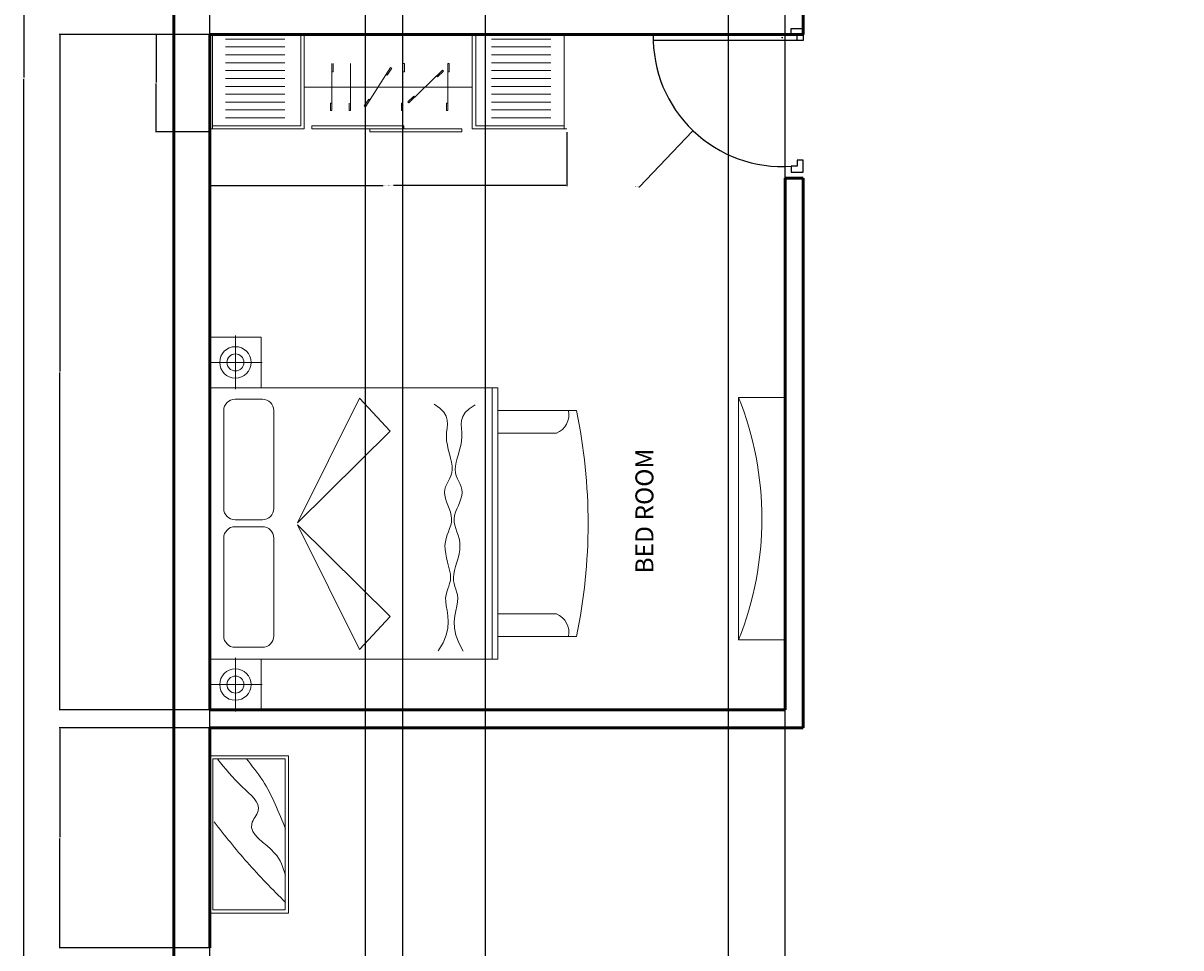
# Model space of a CAD drawing. Units: inches. Extents: x 1865 to 2541, y 1997 to 2759.
# Tile 2 of 11: x 1866 to 2155, y 2174 to 2405. Entities that reach past the tile are written whole.
import ezdxf

# ---------------------------------------------------------------- set-up
doc = ezdxf.new("R2010")
doc.units = ezdxf.units.IN
for name, color, linetype, lineweight in [('A-ANNO-DIMS', 2, 'Continuous', 18), ('A-AREA-IDEN', 4, 'Continuous', 18), ('A-FURN', 8, 'Continuous', 13), ('A-WALL', 7, 'Continuous', 50), ('BED', 42, 'Continuous', 13), ('CUPBOARD', 61, 'Continuous', 18), ('DOOR', 1, 'Continuous', 25), ('TV', 3, 'Continuous', 18)]:
    doc.layers.add(name, color=color, linetype=linetype, lineweight=lineweight)
doc.styles.get("Standard").update_dxf_attribs({"font": 'arial.ttf'})
doc.dimstyles.get("Standard").update_dxf_attribs({"dimtxt": 0.18, "dimasz": 0.18, "dimexe": 0.18, "dimexo": 0.0625, "dimgap": 0.09, "dimtad": 0, "dimtih": 1, "dimtoh": 1, "dimdec": 4, "dimzin": 0, "dimdsep": 46, "dimtxsty": 'Standard', "dimcen": 0.09, "dimadec": 0, "dimazin": 0, "dimtfac": 1, "dimtdec": 4, "dimtofl": 0, "dimtmove": 0, "dimatfit": 3, "dimfxl": 1, "dimtolj": 1, "dimtzin": 0, "dimarcsym": 0})

# ---------------------------------------------------------------- blocks, each defined once
blk = doc.blocks.new('A$C4F543DC7')
for p, q in [((0.013, 3.35, -0.169), (3.313, 3.35, -0.169)), ((0.463, 3.35, -0.169), (0.013, 3.35, -0.169)), ((0.013, 2.896, -0.169), (0.013, 3.35, -0.169)), ((0.013, 3.35, -0.169), (0.013, 2.896, -0.169)), ((0.238, 3.123, -0.439), (0.238, 3.361, -0.439)), ((0.463, 3.35, -0.169), (0.463, 0.8, -0.169)), ((2.863, 3.35, -0.169), (0.463, 3.35, -0.169)), ((0.463, 2.896, -0.169), (0.463, 3.35, -0.169)), ((2.863, 0.8, -0.169), (2.863, 3.35, -0.169)), ((2.863, 3.35, -0.169), (3.313, 3.35, -0.169)), ((2.863, 2.896, -0.169), (2.863, 3.35, -0.169)), ((3.089, 3.123, -0.439), (3.089, 3.361, -0.439)), ((3.313, 3.35, -0.169), (3.313, 2.896, -0.169)), ((3.313, 3.35, -0.169), (3.313, 2.896, -0.169)), ((1.535, 3.226, -0.169), (0.668, 3.226, -0.169)), ((2.664, 3.226, -0.169), (1.797, 3.226, -0.169)), ((0.238, 3.123, -0.439), (0, 3.123, -0.439)), ((0.238, 3.123, -0.439), (0.476, 3.123, -0.439)), ((0.238, 3.123, -0.439), (0.238, 2.885, -0.439)), ((0.568, 3.126, -0.169), (0.568, 2.884, -0.169)), ((1.635, 2.884, -0.169), (1.635, 3.126, -0.169)), ((1.697, 3.126, -0.169), (1.697, 2.884, -0.169)), ((2.764, 2.884, -0.169), (2.764, 3.126, -0.169)), ((3.089, 3.123, -0.439), (2.851, 3.123, -0.439)), ((3.089, 3.123, -0.439), (3.089, 2.885, -0.439)), ((3.089, 3.123, -0.439), (3.327, 3.123, -0.439)), ((0.463, 2.896, -0.169), (0.013, 2.896, -0.169)), ((0.013, 2.896, -0.169), (0.463, 2.896, -0.169)), ((0.463, 0.8, -0.169), (0.463, 2.896, -0.169)), ((2.863, 2.896, -0.169), (2.863, 0.8, -0.169)), ((3.313, 2.896, -0.169), (2.863, 2.896, -0.169)), ((3.313, 2.896, -0.169), (2.863, 2.896, -0.169)), ((0.668, 2.784, -0.169), (1.535, 2.784, -0.169)), ((1.797, 2.784, -0.169), (2.664, 2.784, -0.169)), ((1.653, 2.573, -0.169), (0.55, 2.025, -0.169)), ((0.841, 1.752, -0.169), (1.653, 2.573, -0.169)), ((2.481, 1.752, -0.169), (1.669, 2.573, -0.169)), ((1.669, 2.573, -0.169), (2.772, 2.025, -0.169)), ((0.55, 2.025, -0.169), (0.841, 1.752, -0.169)), ((2.772, 2.025, -0.169), (2.481, 1.752, -0.169)), ((2.683, 1.312, -0.169), (2.718, 1.364, -0.169)), ((0.537, 1.327, -0.169), (0.609, 1.284, -0.169)), ((0.609, 1.284, -0.169), (0.676, 1.257, -0.169)), ((0.676, 1.257, -0.169), (0.737, 1.243, -0.169)), ((0.737, 1.243, -0.169), (0.794, 1.239, -0.169)), ((0.794, 1.239, -0.169), (0.846, 1.242, -0.169)), ((0.846, 1.242, -0.169), (0.893, 1.249, -0.169)), ((0.893, 1.249, -0.169), (0.935, 1.256, -0.169)), ((0.935, 1.256, -0.169), (0.972, 1.261, -0.169)), ((0.972, 1.261, -0.169), (1.004, 1.262, -0.169)), ((1.004, 1.262, -0.169), (1.033, 1.258, -0.169)), ((1.033, 1.258, -0.169), (1.06, 1.251, -0.169)), ((1.06, 1.251, -0.169), (1.084, 1.242, -0.169)), ((1.084, 1.242, -0.169), (1.108, 1.234, -0.169)), ((1.108, 1.234, -0.169), (1.132, 1.226, -0.169)), ((1.25, 1.226, -0.169), (1.285, 1.235, -0.169)), ((1.285, 1.235, -0.169), (1.322, 1.244, -0.169)), ((1.322, 1.244, -0.169), (1.359, 1.253, -0.169)), ((1.359, 1.253, -0.169), (1.396, 1.261, -0.169)), ((1.396, 1.261, -0.169), (1.433, 1.266, -0.169)), ((1.433, 1.266, -0.169), (1.468, 1.268, -0.169)), ((1.468, 1.268, -0.169), (1.501, 1.264, -0.169)), ((1.501, 1.264, -0.169), (1.532, 1.257, -0.169)), ((1.532, 1.257, -0.169), (1.562, 1.247, -0.169)), ((1.562, 1.247, -0.169), (1.591, 1.237, -0.169)), ((1.591, 1.237, -0.169), (1.62, 1.226, -0.169)), ((1.765, 1.22, -0.169), (1.795, 1.23, -0.169)), ((1.795, 1.23, -0.169), (1.826, 1.242, -0.169)), ((1.826, 1.242, -0.169), (1.856, 1.253, -0.169)), ((1.856, 1.253, -0.169), (1.885, 1.263, -0.169)), ((1.885, 1.263, -0.169), (1.913, 1.27, -0.169)), ((1.913, 1.27, -0.169), (1.94, 1.272, -0.169)), ((1.94, 1.272, -0.169), (1.965, 1.269, -0.169)), ((1.965, 1.269, -0.169), (1.989, 1.262, -0.169)), ((1.989, 1.262, -0.169), (2.012, 1.251, -0.169)), ((2.012, 1.251, -0.169), (2.036, 1.239, -0.169)), ((2.036, 1.239, -0.169), (2.06, 1.227, -0.169)), ((2.279, 1.228, -0.169), (2.317, 1.238, -0.169)), ((2.317, 1.238, -0.169), (2.356, 1.246, -0.169)), ((2.356, 1.246, -0.169), (2.394, 1.253, -0.169)), ((2.394, 1.253, -0.169), (2.433, 1.255, -0.169)), ((2.433, 1.255, -0.169), (2.47, 1.253, -0.169)), ((2.47, 1.253, -0.169), (2.506, 1.249, -0.169)), ((2.506, 1.249, -0.169), (2.542, 1.246, -0.169)), ((2.542, 1.246, -0.169), (2.578, 1.248, -0.169)), ((2.578, 1.248, -0.169), (2.613, 1.257, -0.169)), ((2.613, 1.257, -0.169), (2.648, 1.277, -0.169)), ((2.648, 1.277, -0.169), (2.683, 1.312, -0.169)), ((0.533, 1.105, -0.169), (0.607, 1.146, -0.169)), ((0.607, 1.146, -0.169), (0.674, 1.171, -0.169)), ((0.674, 1.171, -0.169), (0.736, 1.183, -0.169)), ((0.736, 1.183, -0.169), (0.793, 1.185, -0.169)), ((0.793, 1.185, -0.169), (0.845, 1.18, -0.169)), ((0.845, 1.18, -0.169), (0.891, 1.172, -0.169)), ((0.891, 1.172, -0.169), (0.933, 1.163, -0.169)), ((0.933, 1.163, -0.169), (0.97, 1.156, -0.169)), ((0.97, 1.156, -0.169), (1.003, 1.155, -0.169)), ((1.003, 1.155, -0.169), (1.032, 1.158, -0.169)), ((1.032, 1.158, -0.169), (1.058, 1.164, -0.169)), ((1.058, 1.164, -0.169), (1.083, 1.172, -0.169)), ((1.083, 1.172, -0.169), (1.107, 1.18, -0.169)), ((1.107, 1.18, -0.169), (1.132, 1.187, -0.169)), ((1.132, 1.226, -0.169), (1.158, 1.22, -0.169)), ((1.132, 1.187, -0.169), (1.157, 1.192, -0.169)), ((1.157, 1.192, -0.169), (1.185, 1.193, -0.169)), ((1.158, 1.22, -0.169), (1.185, 1.218, -0.169)), ((1.185, 1.218, -0.169), (1.216, 1.22, -0.169)), ((1.185, 1.193, -0.169), (1.216, 1.19, -0.169)), ((1.216, 1.22, -0.169), (1.25, 1.226, -0.169)), ((1.216, 1.19, -0.169), (1.249, 1.183, -0.169)), ((1.249, 1.183, -0.169), (1.284, 1.173, -0.169)), ((1.284, 1.173, -0.169), (1.321, 1.163, -0.169)), ((1.321, 1.163, -0.169), (1.358, 1.152, -0.169)), ((1.358, 1.152, -0.169), (1.394, 1.143, -0.169)), ((1.394, 1.143, -0.169), (1.431, 1.137, -0.169)), ((1.431, 1.137, -0.169), (1.466, 1.135, -0.169)), ((1.466, 1.135, -0.169), (1.499, 1.137, -0.169)), ((1.499, 1.137, -0.169), (1.531, 1.143, -0.169)), ((1.531, 1.143, -0.169), (1.561, 1.152, -0.169)), ((1.561, 1.152, -0.169), (1.59, 1.162, -0.169)), ((1.59, 1.162, -0.169), (1.619, 1.172, -0.169)), ((1.619, 1.172, -0.169), (1.648, 1.18, -0.169)), ((1.62, 1.226, -0.169), (1.648, 1.217, -0.169)), ((1.648, 1.217, -0.169), (1.676, 1.211, -0.169)), ((1.648, 1.18, -0.169), (1.676, 1.185, -0.169)), ((1.676, 1.211, -0.169), (1.705, 1.209, -0.169)), ((1.676, 1.185, -0.169), (1.705, 1.186, -0.169)), ((1.705, 1.209, -0.169), (1.735, 1.212, -0.169)), ((1.705, 1.186, -0.169), (1.734, 1.182, -0.169)), ((1.734, 1.182, -0.169), (1.764, 1.173, -0.169)), ((1.735, 1.212, -0.169), (1.765, 1.22, -0.169)), ((1.764, 1.173, -0.169), (1.794, 1.162, -0.169)), ((1.794, 1.162, -0.169), (1.824, 1.149, -0.169)), ((1.824, 1.149, -0.169), (1.854, 1.137, -0.169)), ((1.854, 1.137, -0.169), (1.883, 1.126, -0.169)), ((1.987, 1.124, -0.169), (2.011, 1.134, -0.169)), ((2.011, 1.134, -0.169), (2.034, 1.145, -0.169)), ((2.034, 1.145, -0.169), (2.059, 1.157, -0.169)), ((2.059, 1.157, -0.169), (2.084, 1.167, -0.169)), ((2.06, 1.227, -0.169), (2.085, 1.216, -0.169)), ((2.084, 1.167, -0.169), (2.111, 1.174, -0.169)), ((2.085, 1.216, -0.169), (2.112, 1.208, -0.169)), ((2.111, 1.174, -0.169), (2.14, 1.177, -0.169)), ((2.112, 1.208, -0.169), (2.141, 1.204, -0.169)), ((2.14, 1.177, -0.169), (2.172, 1.175, -0.169)), ((2.141, 1.204, -0.169), (2.172, 1.205, -0.169)), ((2.172, 1.205, -0.169), (2.206, 1.21, -0.169)), ((2.172, 1.175, -0.169), (2.206, 1.169, -0.169)), ((2.206, 1.21, -0.169), (2.242, 1.218, -0.169)), ((2.206, 1.169, -0.169), (2.241, 1.16, -0.169)), ((2.241, 1.16, -0.169), (2.278, 1.149, -0.169)), ((2.242, 1.218, -0.169), (2.279, 1.228, -0.169)), ((2.278, 1.149, -0.169), (2.316, 1.138, -0.169)), ((2.316, 1.138, -0.169), (2.354, 1.128, -0.169)), ((2.354, 1.128, -0.169), (2.392, 1.121, -0.169)), ((1.883, 1.126, -0.169), (1.911, 1.119, -0.169)), ((1.911, 1.119, -0.169), (1.937, 1.115, -0.169)), ((1.937, 1.115, -0.169), (1.963, 1.118, -0.169)), ((1.963, 1.118, -0.169), (1.987, 1.124, -0.169)), ((2.392, 1.121, -0.169), (2.43, 1.117, -0.169)), ((2.43, 1.117, -0.169), (2.468, 1.118, -0.169)), ((2.468, 1.118, -0.169), (2.504, 1.121, -0.169)), ((2.504, 1.121, -0.169), (2.54, 1.123, -0.169)), ((2.54, 1.123, -0.169), (2.576, 1.12, -0.169)), ((2.576, 1.12, -0.169), (2.611, 1.109, -0.169)), ((2.611, 1.109, -0.169), (2.645, 1.088, -0.169)), ((2.645, 1.088, -0.169), (2.679, 1.052, -0.169)), ((2.679, 1.052, -0.169), (2.712, 0.999, -0.169)), ((0.463, 0.85, -0.169), (2.863, 0.85, -0.169)), ((0.463, 0.8, -0.169), (2.863, 0.8, -0.169)), ((0.663, 0.8, -0.169), (0.463, 0.8, -0.169)), ((0.663, 0.8, -0.169), (2.663, 0.8, -0.169)), ((0.663, 0.104, -0.169), (0.663, 0.8, -0.169)), ((0.663, 0.104, -0.169), (0.663, 0.8, -0.169)), ((0.863, 0.281, -0.169), (0.863, 0.8, -0.169)), ((2.463, 0.8, -0.169), (2.463, 0.281, -0.169)), ((2.863, 0.8, -0.169), (2.663, 0.8, -0.169)), ((2.663, 0.8, -0.169), (2.663, 0.104, -0.169)), ((2.663, 0.8, -0.169), (2.663, 0.104, -0.169))]:
    blk.add_line(p, q)
for centre, radius in [((0.238, 3.123, -0.439), 0.139), ((0.238, 3.123, -0.439), 0.075), ((3.089, 3.123, -0.439), 0.139), ((3.089, 3.123, -0.439), 0.075)]:
    blk.add_circle(centre, radius)
for centre, radius, start, end in [((0.668, 3.126, -0.169), 0.1, 90, 180), ((1.535, 3.126, -0.169), 0.1, 0, 90), ((1.797, 3.126, -0.169), 0.1, 90, 180), ((2.664, 3.126, -0.169), 0.1, 0, 90), ((0.668, 2.884, -0.169), 0.1, 180, 270), ((1.535, 2.884, -0.169), 0.1, 270, 0), ((1.797, 2.884, -0.169), 0.1, 180, 270), ((2.664, 2.884, -0.169), 0.1, 270, 0), ((0.699, 0.347, -0.169), 0.177, 258.2616, 338.032), ((2.627, 0.347, -0.169), 0.177, 201.968, 281.7384), ((1.663, 4.86, -0.169), 4.86, 258.1252, 281.8748), ((1.663, 4.86, -0.169), 4.86, 258.1252, 281.8748)]:
    blk.add_arc(centre, radius, start, end)
blk = doc.blocks.new('A$C34930FF8')
at = {"ltscale": 0.05}
for p, q in [((0, 2252.4), (0, 16.8)), ((600, 2252.4), (0, 2252.4)), ((185.4, 1513), (185.4, 1521.5)), ((227.1, 1479.2), (233.2, 1485.2)), ((237.7, 1513), (237.7, 1521.5)), ((436.7, 1513), (436.7, 1504.4)), ((482.5, 1513), (482.5, 1504.4)), ((263.6, 1441.7), (269.7, 1447.7)), ((398.2, 1303.6), (392.1, 1297.6)), ((434.8, 1266.1), (428.7, 1260.1)), ((185.4, 1229.1), (185.4, 1237.7)), ((237.7, 1229.1), (237.7, 1237.7)), ((436.7, 1228.2), (436.7, 1219.7)), ((482.5, 1228.2), (482.5, 1219.7)), ((209.5, 1150.1), (214.1, 1157.3)), ((253.5, 1121.8), (258.1, 1129)), ((415.3, 1017.6), (410.6, 1010.5)), ((459.3, 989.3), (454.7, 982.1)), ((482.5, 894.9), (482.5, 886.3)), ((237.7, 775.3), (237.7, 783.9)), ((436.7, 775.3), (436.7, 766.8)), ((482.5, 775.3), (482.5, 766.8)), ((600, 16.8), (0, 16.8))]:
    blk.add_line(p, q, dxfattribs=at)
for p, q in [((580, 1690.9), (580, 2252.4)), ((600, 1669.3), (600, 2269.3)), ((30, 1790.9), (30, 2169.3)), ((80, 1790.9), (80, 2169.3)), ((130, 1790.9), (130, 2169.3)), ((180, 1790.9), (180, 2169.3)), ((230, 1790.9), (230, 2169.3)), ((280, 1790.9), (280, 2169.3)), ((330, 1790.9), (330, 2169.3)), ((380, 1790.9), (380, 2169.3)), ((430, 1790.9), (430, 2169.3)), ((480, 1790.9), (480, 2169.3)), ((530, 1790.9), (530, 2169.3)), ((580, 1690.9), (0, 1690.9)), ((600, 1669.3), (0, 1669.3)), ((335.4, 1666.1), (335.4, 603.1)), ((600, 1603.3), (620, 1603.3)), ((600, 1018.7), (600, 1603.3)), ((620, 1603.3), (620, 1018.7)), ((237.7, 1521.5), (185.4, 1521.5)), ((482.5, 1513), (185.4, 1513)), ((434.8, 1266.1), (227.4, 1478.9)), ((269.7, 1447.7), (233.2, 1485.2)), ((436.7, 1504.4), (482.5, 1504.4)), ((428.7, 1260.1), (392.1, 1297.6)), ((237.7, 1237.7), (185.4, 1237.7)), ((482.5, 1228.2), (185.4, 1228.2)), ((436.7, 1219.7), (482.5, 1219.7)), ((600, 1233.4), (580, 1233.4)), ((580, 1233.4), (580, 648.7)), ((600, 648.7), (600, 1233.4)), ((459.3, 989.3), (209.5, 1150.1)), ((258.1, 1129), (214.1, 1157.3)), ((454.7, 982.1), (410.6, 1010.5)), ((620, 1018.7), (600, 1018.7)), ((482.5, 894.9), (185.4, 894.9)), ((436.7, 886.3), (482.5, 886.3)), ((237.7, 783.9), (185.4, 783.9)), ((482.5, 775.3), (185.4, 775.3)), ((436.7, 766.8), (482.5, 766.8)), ((600, 600), (0, 600)), ((580, 648.7), (600, 648.7)), ((600, 600), (600, 0)), ((580, 578.3), (0, 578.3)), ((580, 578.3), (580, 16.8)), ((30, 478.3), (30, 100)), ((80, 478.3), (80, 100)), ((130, 478.3), (130, 100)), ((180, 478.3), (180, 100)), ((230, 478.3), (230, 100)), ((280, 478.3), (280, 100)), ((330, 478.3), (330, 100)), ((380, 478.3), (380, 100)), ((430, 478.3), (430, 100)), ((480, 478.3), (480, 100)), ((530, 478.3), (530, 100))]:
    blk.add_line(p, q)
blk = doc.blocks.new('DOOR-SWING-36IN')
for p, q in [((34.51, 36), (37.51, 36)), ((34.51, 34.5), (34.51, 36)), ((37.51, 36), (37.51, 33)), ((36.01, 34.5), (0.01, 34.5)), ((36.01, 33), (0.01, 33)), ((36.01, 34.5), (34.51, 34.5)), ((36.01, 33), (36.01, 34.5)), ((37.51, 33), (36.01, 33)), ((37.51, 3), (36.01, 3)), ((36.01, 3), (36.01, 1.5)), ((37.51, 0), (37.51, 3)), ((36.01, 1.5), (34.51, 1.5)), ((34.51, 1.5), (34.51, 0)), ((34.51, 0), (37.51, 0))]:
    blk.add_line(p, q)
blk.add_arc((32.32, 33.75), 32.32, 178.6705, 273.8756)
blk = doc.blocks.new('TABLE-COFFEE-RECT')
for p, q in [((0, 39.37), (0, 0)), ((19.69, 39.37), (0, 39.37)), ((0.79, 38.58), (0.79, 0.79)), ((18.9, 38.58), (0.79, 38.58)), ((18.9, 0.79), (18.9, 38.58)), ((19.69, 0), (19.69, 39.37)), ((0.79, 0.79), (18.9, 0.79)), ((0, 0), (19.69, 0))]:
    blk.add_line(p, q)
for points, knots in [([(18.6, 16.56), (15.9, 19.98), (10.33, 27.05), (3.98, 33.45), (0.7, 36.75)], [0, 0, 0, 0, 13.044093, 27.000677, 27.000677, 27.000677, 27.000677]), ([(17.68, 0.96), (15.88, 3.19), (12.68, 7.14), (5.8, 12.67), (11.59, 18.88), (2.91, 23.18), (1.33, 27.96), (0.7, 29.87)], [0, 0, 0, 0, 9.260592, 16.388167, 19.979545, 29.29681, 35.453459, 35.453459, 35.453459, 35.453459]), ([(10.57, 0.73), (9.12, 2.52), (4.86, 7.82), (2.36, 14.19), (0.7, 18.4)], [0, 0, 0, 0, 6.883342, 20.328879, 20.328879, 20.328879, 20.328879])]:
    blk.add_open_spline(points, degree=3, knots=knots)
blk = doc.blocks.new('TV-UNIT')
blk.add_lwpolyline([(0, 11.62), (60.65, 11.62), (60.65, 0), (0, 0)], close=True)
blk.add_arc((30.32, -76.26), 82.06, 68.3146, 111.6854)
blk = doc.blocks.new('*D26')
at = {"layer": 'A-ANNO-DIMS', "color": 0, "lineweight": -2, "transparency": 16777216}
for p, q in [((1912.24, 2377.98), (1912.24, 2364.46)), ((2001.58, 2377.98), (2001.58, 2364.46)), ((1912.42, 2364.64), (1955.61, 2364.64)), ((2001.4, 2364.64), (1958.22, 2364.64))]:
    blk.add_line(p, q, dxfattribs=at)
at = {"layer": 'A-ANNO-DIMS', "color": 0, "transparency": 16777216}
for points in [[(1912.42, 2364.67), (1912.42, 2364.61), (1912.24, 2364.64)], [(2001.4, 2364.67), (2001.4, 2364.61), (2001.58, 2364.64)]]:
    blk.add_solid(points, dxfattribs=at)
at = {"layer": 'Defpoints', "color": 0, "transparency": 16777216}
for p in [(1912.24, 2378.04), (2001.58, 2378.04), (2001.58, 2364.64)]:
    blk.add_point(p, dxfattribs=at)
at = {"layer": 'A-ANNO-DIMS', "color": 0, "transparency": 16777216, "insert": (1956.91, 2364.64), "char_height": 0.18, "attachment_point": 5}
blk.add_mtext('\\A1;WARDROBE 89 TYP.', dxfattribs=at)
blk = doc.blocks.new('*D27')
at = {"layer": 'A-ANNO-DIMS', "color": 0, "lineweight": -2, "transparency": 16777216}
for p, q in [((1912.18, 2402.45), (1898.66, 2402.45)), ((1898.84, 2402.27), (1898.84, 2390.43)), ((1898.84, 2378.22), (1898.84, 2390.06)), ((1912.18, 2378.04), (1898.66, 2378.04))]:
    blk.add_line(p, q, dxfattribs=at)
at = {"layer": 'A-ANNO-DIMS', "color": 0, "transparency": 16777216}
for points in [[(1898.81, 2402.27), (1898.87, 2402.27), (1898.84, 2402.45)], [(1898.81, 2378.22), (1898.87, 2378.22), (1898.84, 2378.04)]]:
    blk.add_solid(points, dxfattribs=at)
at = {"layer": 'Defpoints', "color": 0, "transparency": 16777216}
for p in [(1912.24, 2402.45), (1898.84, 2378.04), (1912.24, 2378.04)]:
    blk.add_point(p, dxfattribs=at)
at = {"layer": 'A-ANNO-DIMS', "color": 0, "transparency": 16777216, "insert": (1898.84, 2390.24), "char_height": 0.18, "attachment_point": 5}
blk.add_mtext('\\A1;24 TYP.', dxfattribs=at)
blk = doc.blocks.new('*D41')
at = {"layer": 'A-ANNO-DIMS', "color": 0, "lineweight": -2, "transparency": 16777216}
for p, q in [((2503.31, 2721.45), (2540.92, 2721.45)), ((2540.74, 2721.27), (2540.74, 2378.49)), ((2540.74, 2035.35), (2540.74, 2378.13)), ((2136.19, 2035.17), (2540.92, 2035.17))]:
    blk.add_line(p, q, dxfattribs=at)
at = {"layer": 'A-ANNO-DIMS', "color": 0, "transparency": 16777216}
for points in [[(2540.71, 2721.27), (2540.77, 2721.27), (2540.74, 2721.45)], [(2540.71, 2035.35), (2540.77, 2035.35), (2540.74, 2035.17)]]:
    blk.add_solid(points, dxfattribs=at)
at = {"layer": 'Defpoints', "color": 0, "transparency": 16777216}
for p in [(2503.24, 2721.45), (2136.13, 2035.17), (2540.74, 2035.17)]:
    blk.add_point(p, dxfattribs=at)
at = {"layer": 'A-ANNO-DIMS', "color": 0, "transparency": 16777216, "insert": (2540.74, 2378.31), "char_height": 0.18, "attachment_point": 5}
blk.add_mtext('\\A1;686.3', dxfattribs=at)
blk = doc.blocks.new('*D42')
at = {"layer": 'A-ANNO-DIMS', "color": 0, "lineweight": -2, "transparency": 16777216}
for p, q in [((1903.18, 2721.45), (1865.56, 2721.45)), ((1865.74, 2721.27), (1865.74, 2391.63)), ((1865.74, 2061.63), (1865.74, 2391.27)), ((1903.18, 2061.45), (1865.56, 2061.45))]:
    blk.add_line(p, q, dxfattribs=at)
at = {"layer": 'A-ANNO-DIMS', "color": 0, "transparency": 16777216}
for points in [[(1865.71, 2721.27), (1865.77, 2721.27), (1865.74, 2721.45)], [(1865.71, 2061.63), (1865.77, 2061.63), (1865.74, 2061.45)]]:
    blk.add_solid(points, dxfattribs=at)
at = {"layer": 'Defpoints', "color": 0, "transparency": 16777216}
for p in [(1865.74, 2721.45), (1903.24, 2721.45), (1903.24, 2061.45)]:
    blk.add_point(p, dxfattribs=at)
at = {"layer": 'A-ANNO-DIMS', "color": 0, "transparency": 16777216, "insert": (1865.74, 2391.45), "char_height": 0.18, "attachment_point": 5}
blk.add_mtext('\\A1;660', dxfattribs=at)
blk = doc.blocks.new('*D49')
at = {"layer": 'A-ANNO-DIMS', "color": 0, "lineweight": -2, "transparency": 16777216}
for p, q in [((1912.18, 2402.45), (1874.56, 2402.45)), ((1874.74, 2402.27), (1874.74, 2318.13)), ((1874.74, 2233.63), (1874.74, 2317.77)), ((1912.18, 2233.45), (1874.56, 2233.45))]:
    blk.add_line(p, q, dxfattribs=at)
at = {"layer": 'A-ANNO-DIMS', "color": 0, "transparency": 16777216}
for points in [[(1874.71, 2402.27), (1874.77, 2402.27), (1874.74, 2402.45)], [(1874.71, 2233.63), (1874.77, 2233.63), (1874.74, 2233.45)]]:
    blk.add_solid(points, dxfattribs=at)
at = {"layer": 'Defpoints', "color": 0, "transparency": 16777216}
for p in [(1874.74, 2402.45), (1912.24, 2402.45), (1912.24, 2233.45)]:
    blk.add_point(p, dxfattribs=at)
at = {"layer": 'A-ANNO-DIMS', "color": 0, "transparency": 16777216, "insert": (1874.74, 2317.95), "char_height": 0.18, "attachment_point": 5}
blk.add_mtext('\\A1;169', dxfattribs=at)
blk = doc.blocks.new('*D50')
at = {"layer": 'A-ANNO-DIMS', "color": 0, "lineweight": -2, "transparency": 16777216}
for p, q in [((1912.18, 2228.95), (1874.56, 2228.95)), ((1874.74, 2228.77), (1874.74, 2201.63)), ((1874.74, 2174.13), (1874.74, 2201.27)), ((1912.18, 2173.95), (1874.56, 2173.95))]:
    blk.add_line(p, q, dxfattribs=at)
at = {"layer": 'A-ANNO-DIMS', "color": 0, "transparency": 16777216}
for points in [[(1874.71, 2228.77), (1874.77, 2228.77), (1874.74, 2228.95)], [(1874.71, 2174.13), (1874.77, 2174.13), (1874.74, 2173.95)]]:
    blk.add_solid(points, dxfattribs=at)
at = {"layer": 'Defpoints', "color": 0, "transparency": 16777216}
for p in [(1874.74, 2228.95), (1912.24, 2228.95), (1912.24, 2173.95)]:
    blk.add_point(p, dxfattribs=at)
at = {"layer": 'A-ANNO-DIMS', "color": 0, "transparency": 16777216, "insert": (1874.74, 2201.45), "char_height": 0.18, "attachment_point": 5}
blk.add_mtext('\\A1;55', dxfattribs=at)
blk = doc.blocks.new('*D68')
at = {"layer": 'A-ANNO-DIMS', "color": 0, "lineweight": -2, "transparency": 16777216}
for p, q in [((1912.24, 2169.51), (1912.24, 2759.13)), ((1912.42, 2758.95), (1931.52, 2758.95)), ((1951.06, 2758.95), (1931.96, 2758.95)), ((1951.24, 2169.51), (1951.24, 2759.13))]:
    blk.add_line(p, q, dxfattribs=at)
at = {"layer": 'A-ANNO-DIMS', "color": 0, "transparency": 16777216}
for points in [[(1912.42, 2758.98), (1912.42, 2758.92), (1912.24, 2758.95)], [(1951.06, 2758.98), (1951.06, 2758.92), (1951.24, 2758.95)]]:
    blk.add_solid(points, dxfattribs=at)
at = {"layer": 'Defpoints', "color": 0, "transparency": 16777216}
for p in [(1951.24, 2758.95), (1912.24, 2169.45), (1951.24, 2169.45)]:
    blk.add_point(p, dxfattribs=at)
at = {"layer": 'A-ANNO-DIMS', "color": 0, "transparency": 16777216, "insert": (1931.74, 2758.95), "char_height": 0.18, "attachment_point": 5}
blk.add_mtext('\\A1;39', dxfattribs=at)
blk = doc.blocks.new('*D81')
at = {"layer": 'A-ANNO-DIMS', "color": 0, "lineweight": -2, "transparency": 16777216}
for p, q in [((1960.58, 2070.51), (1960.58, 2759.13)), ((1960.76, 2758.95), (1970.44, 2758.95)), ((1981.06, 2758.95), (1971.38, 2758.95)), ((1981.24, 2070.51), (1981.24, 2759.13))]:
    blk.add_line(p, q, dxfattribs=at)
at = {"layer": 'A-ANNO-DIMS', "color": 0, "transparency": 16777216}
for points in [[(1960.76, 2758.98), (1960.76, 2758.92), (1960.58, 2758.95)], [(1981.06, 2758.98), (1981.06, 2758.92), (1981.24, 2758.95)]]:
    blk.add_solid(points, dxfattribs=at)
at = {"layer": 'Defpoints', "color": 0, "transparency": 16777216}
for p in [(1960.58, 2758.95), (1960.58, 2070.45), (1981.24, 2070.45)]:
    blk.add_point(p, dxfattribs=at)
at = {"layer": 'A-ANNO-DIMS', "color": 0, "transparency": 16777216, "insert": (1970.91, 2758.95), "char_height": 0.18, "attachment_point": 5}
blk.add_mtext('\\A1;20.665', dxfattribs=at)
blk = doc.blocks.new('*D82')
at = {"layer": 'A-ANNO-DIMS', "color": 0, "lineweight": -2, "transparency": 16777216}
for p, q in [((2042.07, 2070.51), (2042.07, 2759.13)), ((2042.25, 2758.95), (2048.7, 2758.95)), ((2056.06, 2758.95), (2049.61, 2758.95)), ((2056.24, 2070.51), (2056.24, 2759.13))]:
    blk.add_line(p, q, dxfattribs=at)
at = {"layer": 'A-ANNO-DIMS', "color": 0, "transparency": 16777216}
for points in [[(2042.25, 2758.98), (2042.25, 2758.92), (2042.07, 2758.95)], [(2056.06, 2758.98), (2056.06, 2758.92), (2056.24, 2758.95)]]:
    blk.add_solid(points, dxfattribs=at)
at = {"layer": 'Defpoints', "color": 0, "transparency": 16777216}
for p in [(2042.07, 2758.95), (2042.07, 2070.45), (2056.24, 2070.45)]:
    blk.add_point(p, dxfattribs=at)
at = {"layer": 'A-ANNO-DIMS', "color": 0, "transparency": 16777216, "insert": (2049.16, 2758.95), "char_height": 0.18, "attachment_point": 5}
blk.add_mtext('\\A1;14.176', dxfattribs=at)
blk = doc.blocks.new('*D86')
at = {"layer": 'A-ANNO-DIMS', "color": 0, "lineweight": -2, "transparency": 16777216}
for p, q in [((2055.47, 2401.7), (2055.65, 2401.7)), ((2055.56, 2401.61), (2055.56, 2401.79)), ((2019.81, 2364.33), (2033.09, 2378.21)), ((2019.63, 2364.33), (2019.81, 2364.33))]:
    blk.add_line(p, q, dxfattribs=at)
at = {"layer": 'A-ANNO-DIMS', "color": 0, "transparency": 16777216}
blk.add_solid([(2033.07, 2378.23), (2033.11, 2378.19), (2033.21, 2378.34)], dxfattribs=at)
at = {"layer": 'Defpoints', "color": 0, "transparency": 16777216}
for p in [(2055.56, 2401.7), (2033.21, 2378.34)]:
    blk.add_point(p, dxfattribs=at)
at = {"layer": 'A-ANNO-DIMS', "color": 0, "transparency": 16777216, "insert": (2019.08, 2364.33), "char_height": 0.18, "attachment_point": 5}
blk.add_mtext('\\A1;R32.324', dxfattribs=at)

msp = doc.modelspace()

# ---------------------------------------------------------------- linework, layer by layer
at = {"layer": 'A-WALL'}
for p, q in [((1903.243, 2721.4494), (1903.243, 2061.4494)), ((2060.743, 2521.9494), (2060.743, 2402.4494)), ((2056.243, 2402.4494), (1912.243, 2402.4494)), ((1912.243, 2402.4494), (1912.243, 2233.4494)), ((2056.243, 2402.4494), (2060.743, 2402.4494)), ((2056.243, 2366.4494), (2056.243, 2233.4494)), ((2056.243, 2366.4494), (2060.743, 2366.4494)), ((2060.743, 2366.4494), (2060.743, 2228.9494)), ((2056.243, 2233.4494), (1912.243, 2233.4494)), ((2056.243, 2228.9494), (1912.243, 2228.9494)), ((1912.243, 2228.9494), (1912.243, 2173.9494)), ((2056.243, 2228.9494), (2060.743, 2228.9494))]:
    msp.add_line(p, q, dxfattribs=at)

# ---------------------------------------------------------------- block references
at = {"layer": 'A-FURN', "rotation": 180}
msp.add_blockref('TABLE-COFFEE-RECT', (1931.9284, 2222.0184), dxfattribs=at)
at = {"layer": 'BED', "xscale": 28.27205529407425, "yscale": 28.27205529407425, "zscale": 28.27205529407425, "rotation": 90}
msp.add_blockref('A$C4F543DC7', (2006.9544, 2233.0695, 4.7709), dxfattribs=at)
at = {"layer": 'CUPBOARD', "xscale": 0.0393700787401575, "yscale": 0.0393700787401575, "zscale": 0.0393700787401575, "rotation": 270}
msp.add_blockref('A$C34930FF8', (1912.243, 2402.4494), dxfattribs=at)
at = {"layer": 'DOOR'}
msp.add_blockref('DOOR-SWING-36IN', (2023.234, 2367.949), dxfattribs=at)
at = {"layer": 'TV', "extrusion": (0, 0, -1), "zscale": -1, "rotation": 89.99999999999991}
msp.add_blockref('TV-UNIT', (-2044.6276, 2250.986), dxfattribs=at)

# ---------------------------------------------------------------- texts
at = {"layer": 'A-AREA-IDEN', "insert": (2018.7823, 2267.5856), "char_height": 4.5, "attachment_point": 1, "rotation": 90}
msp.add_mtext_dynamic_manual_height_columns('BED ROOM', width=66.075761, gutter_width=12.5, heights=[0], dxfattribs=at)

# ---------------------------------------------------------------- dimensions: what is measured, and where the dimension line sits
at = {"layer": 'A-ANNO-DIMS'}
for base, p1, p2, override, picture, middle in [((1951.243, 2758.9494), (1912.243, 2169.4494), (1951.243, 2169.4494), {"dimdec": 0, "dimlfac": 1, "dimrnd": 0, "dimzin": 0, "dimdsep": 46, "dimlunit": 2}, '*D68', (1931.743, 2758.9494)), ((1960.57848, 2758.94943), (1981.243, 2070.44943), (1960.57848, 2070.44943), {"dimdec": 3, "dimlfac": 1, "dimrnd": 0, "dimzin": 0, "dimdsep": 46, "dimlunit": 2}, '*D81', (1970.91074, 2758.94943)), ((2042.0671, 2758.9494), (2056.243, 2070.4494), (2042.0671, 2070.4494), {"dimdec": 3, "dimlfac": 1, "dimrnd": 0, "dimzin": 0, "dimdsep": 46, "dimlunit": 2}, '*D82', (2049.1551, 2758.9494))]:
    dim = msp.add_linear_dim(base=base, p1=p1, p2=p2, dimstyle='Standard', override=override, dxfattribs=at)
    dim.commit()
    dim.dimension.update_dxf_attribs({"geometry": picture, "text_midpoint": middle})
for base, p1, p2, override, picture, middle in [((1865.743, 2721.4494), (1903.243, 2061.4494), (1903.243, 2721.4494), {"dimdec": 0, "dimlfac": 1, "dimrnd": 0, "dimzin": 0, "dimdsep": 46, "dimlunit": 2}, '*D42', (1865.743, 2391.4494)), ((2540.743, 2035.1708), (2503.243, 2721.4494), (2136.13, 2035.1708), {"dimdec": 1, "dimlfac": 1, "dimrnd": 0, "dimzin": 0, "dimdsep": 46, "dimlunit": 2}, '*D41', (2540.743, 2378.3101)), ((1874.743, 2402.4494), (1912.243, 2233.4494), (1912.243, 2402.4494), {"dimdec": 0, "dimlfac": 1, "dimrnd": 0, "dimzin": 0, "dimdsep": 46, "dimlunit": 2}, '*D49', (1874.743, 2317.9494)), ((1874.743, 2228.9494), (1912.243, 2173.9494), (1912.243, 2228.9494), {"dimdec": 0, "dimlfac": 1, "dimrnd": 0, "dimzin": 0, "dimdsep": 46, "dimlunit": 2}, '*D50', (1874.743, 2201.4494))]:
    dim = msp.add_linear_dim(base=base, p1=p1, p2=p2, angle=90, dimstyle='Standard', override=override, dxfattribs=at)
    dim.commit()
    dim.dimension.update_dxf_attribs({"geometry": picture, "text_midpoint": middle})
dim = msp.add_linear_dim(base=(1898.8418, 2378.04), p1=(1912.243, 2402.4494), p2=(1912.243, 2378.04), angle=270, text='<> TYP.', dimstyle='Standard', override={"dimdec": 0, "dimlfac": 1, "dimrnd": 0, "dimzin": 0, "dimdsep": 46, "dimlunit": 2}, dxfattribs=at)
dim.commit()
dim.dimension.update_dxf_attribs({"geometry": '*D27', "text_midpoint": (1898.8418, 2390.2447)})
dim = msp.add_radius_dim(center=(2055.5582, 2401.6994), mpoint=(2033.215, 2378.341), dimstyle='Standard', override={"dimdec": 3, "dimlfac": 1, "dimrnd": 0, "dimzin": 0, "dimdsep": 46, "dimlunit": 2}, dxfattribs=at)
dim.commit()
dim.dimension.update_dxf_attribs({"geometry": '*D86', "text_midpoint": (2019.0797, 2364.3259), "dimtype": 164})
dim = msp.add_linear_dim(base=(2001.5841, 2364.6388), p1=(1912.243, 2378.04), p2=(2001.5841, 2378.04), text='WARDROBE <> TYP.', dimstyle='Standard', override={"dimdec": 0, "dimlfac": 1, "dimrnd": 0, "dimzin": 0, "dimdsep": 46, "dimlunit": 2}, dxfattribs=at)
dim.commit()
dim.dimension.update_dxf_attribs({"geometry": '*D26', "text_midpoint": (1956.9135, 2364.6388)})

doc.saveas('drawing.dxf')
